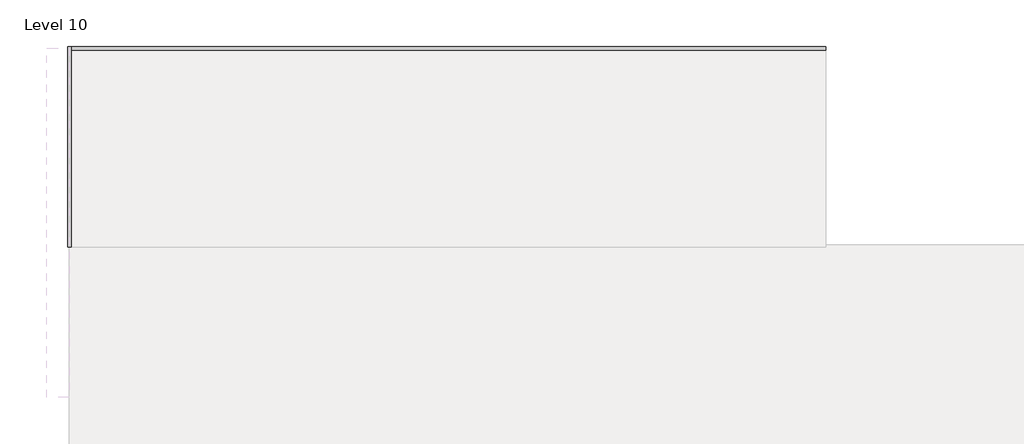
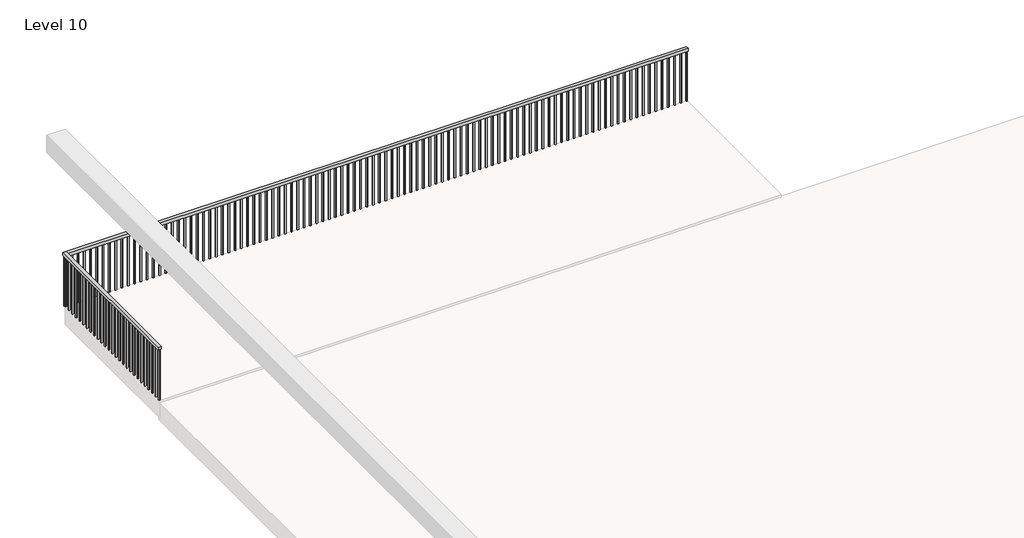
# One storey, part 3 of 5: 2 railings.
"""IFC4 building model written with IfcOpenShell, lengths in millimetres."""

from ifc_helpers import new_model, si_unit, frame, origin, place, context, project, spatial, polyline, outline, extrude, element, save

model = new_model("IFC4")

# Units and contexts
model_context = context("Model", 3, world=origin())
ifc_project = project(units=[si_unit("LENGTHUNIT", "METRE", prefix="MILLI")], contexts=[model_context])

# Site, building, storey
site = spatial("IfcSite", under=ifc_project)
building = spatial("IfcBuilding", under=site)
storey = spatial("IfcBuildingStorey", under=building, Name="Level 10", Elevation=12496.8)

# Railings
placement = place(None, origin())
element("IfcRailing", 1, ObjectType="Handrail - Rectangular", at=placement, inside=storey, context=model_context, shape_type="SweptSolid", body=[
    extrude(outline(polyline([(-13833.4638778, 17386.5959632), (-13833.4638778, 17437.3959632), (-3775.0638778, 17437.3959632), (-3775.0638778, 17386.5959632), (-13833.4638778, 17386.5959632)])), frame((0.0, 0.0, 13360.4), z_axis=(0.0, 0.0, 1.0), x_axis=(1.0, 0.0, 0.0)), (0.0, 0.0, 1.0), 50.8),
    extrude(outline(polyline([(-3886.1888778, 17402.4709632), (-3886.1888778, 17421.5209632), (-3867.1388778, 17421.5209632), (-3867.1388778, 17402.4709632), (-3886.1888778, 17402.4709632)])), frame((0.0, 0.0, 12496.8), z_axis=(0.0, 0.0, 1.0), x_axis=(1.0, 0.0, 0.0)), (0.0, 0.0, 1.0), 863.6),
    extrude(outline(polyline([(-3987.7888778, 17402.4709632), (-3987.7888778, 17421.5209632), (-3968.7388778, 17421.5209632), (-3968.7388778, 17402.4709632), (-3987.7888778, 17402.4709632)])), frame((0.0, 0.0, 12496.8), z_axis=(0.0, 0.0, 1.0), x_axis=(1.0, 0.0, 0.0)), (0.0, 0.0, 1.0), 863.6),
    extrude(outline(polyline([(-4089.3888778, 17402.4709632), (-4089.3888778, 17421.5209632), (-4070.3388778, 17421.5209632), (-4070.3388778, 17402.4709632), (-4089.3888778, 17402.4709632)])), frame((0.0, 0.0, 12496.8), z_axis=(0.0, 0.0, 1.0), x_axis=(1.0, 0.0, 0.0)), (0.0, 0.0, 1.0), 863.6),
    extrude(outline(polyline([(-4190.9888778, 17402.4709632), (-4190.9888778, 17421.5209632), (-4171.9388778, 17421.5209632), (-4171.9388778, 17402.4709632), (-4190.9888778, 17402.4709632)])), frame((0.0, 0.0, 12496.8), z_axis=(0.0, 0.0, 1.0), x_axis=(1.0, 0.0, 0.0)), (0.0, 0.0, 1.0), 863.6),
    extrude(outline(polyline([(-4292.5888778, 17402.4709632), (-4292.5888778, 17421.5209632), (-4273.5388778, 17421.5209632), (-4273.5388778, 17402.4709632), (-4292.5888778, 17402.4709632)])), frame((0.0, 0.0, 12496.8), z_axis=(0.0, 0.0, 1.0), x_axis=(1.0, 0.0, 0.0)), (0.0, 0.0, 1.0), 863.6),
    extrude(outline(polyline([(-4394.1888778, 17402.4709632), (-4394.1888778, 17421.5209632), (-4375.1388778, 17421.5209632), (-4375.1388778, 17402.4709632), (-4394.1888778, 17402.4709632)])), frame((0.0, 0.0, 12496.8), z_axis=(0.0, 0.0, 1.0), x_axis=(1.0, 0.0, 0.0)), (0.0, 0.0, 1.0), 863.6),
    extrude(outline(polyline([(-4495.7888778, 17402.4709632), (-4495.7888778, 17421.5209632), (-4476.7388778, 17421.5209632), (-4476.7388778, 17402.4709632), (-4495.7888778, 17402.4709632)])), frame((0.0, 0.0, 12496.8), z_axis=(0.0, 0.0, 1.0), x_axis=(1.0, 0.0, 0.0)), (0.0, 0.0, 1.0), 863.6),
    extrude(outline(polyline([(-4597.3888778, 17402.4709632), (-4597.3888778, 17421.5209632), (-4578.3388778, 17421.5209632), (-4578.3388778, 17402.4709632), (-4597.3888778, 17402.4709632)])), frame((0.0, 0.0, 12496.8), z_axis=(0.0, 0.0, 1.0), x_axis=(1.0, 0.0, 0.0)), (0.0, 0.0, 1.0), 863.6),
    extrude(outline(polyline([(-4698.9888778, 17402.4709632), (-4698.9888778, 17421.5209632), (-4679.9388778, 17421.5209632), (-4679.9388778, 17402.4709632), (-4698.9888778, 17402.4709632)])), frame((0.0, 0.0, 12496.8), z_axis=(0.0, 0.0, 1.0), x_axis=(1.0, 0.0, 0.0)), (0.0, 0.0, 1.0), 863.6),
    extrude(outline(polyline([(-4800.5888778, 17402.4709632), (-4800.5888778, 17421.5209632), (-4781.5388778, 17421.5209632), (-4781.5388778, 17402.4709632), (-4800.5888778, 17402.4709632)])), frame((0.0, 0.0, 12496.8), z_axis=(0.0, 0.0, 1.0), x_axis=(1.0, 0.0, 0.0)), (0.0, 0.0, 1.0), 863.6),
    extrude(outline(polyline([(-4902.1888778, 17402.4709632), (-4902.1888778, 17421.5209632), (-4883.1388778, 17421.5209632), (-4883.1388778, 17402.4709632), (-4902.1888778, 17402.4709632)])), frame((0.0, 0.0, 12496.8), z_axis=(0.0, 0.0, 1.0), x_axis=(1.0, 0.0, 0.0)), (0.0, 0.0, 1.0), 863.6),
    extrude(outline(polyline([(-5003.7888778, 17402.4709632), (-5003.7888778, 17421.5209632), (-4984.7388778, 17421.5209632), (-4984.7388778, 17402.4709632), (-5003.7888778, 17402.4709632)])), frame((0.0, 0.0, 12496.8), z_axis=(0.0, 0.0, 1.0), x_axis=(1.0, 0.0, 0.0)), (0.0, 0.0, 1.0), 863.6),
    extrude(outline(polyline([(-5105.3888778, 17402.4709632), (-5105.3888778, 17421.5209632), (-5086.3388778, 17421.5209632), (-5086.3388778, 17402.4709632), (-5105.3888778, 17402.4709632)])), frame((0.0, 0.0, 12496.8), z_axis=(0.0, 0.0, 1.0), x_axis=(1.0, 0.0, 0.0)), (0.0, 0.0, 1.0), 863.6),
    extrude(outline(polyline([(-5206.9888778, 17402.4709632), (-5206.9888778, 17421.5209632), (-5187.9388778, 17421.5209632), (-5187.9388778, 17402.4709632), (-5206.9888778, 17402.4709632)])), frame((0.0, 0.0, 12496.8), z_axis=(0.0, 0.0, 1.0), x_axis=(1.0, 0.0, 0.0)), (0.0, 0.0, 1.0), 863.6),
    extrude(outline(polyline([(-5308.5888778, 17402.4709632), (-5308.5888778, 17421.5209632), (-5289.5388778, 17421.5209632), (-5289.5388778, 17402.4709632), (-5308.5888778, 17402.4709632)])), frame((0.0, 0.0, 12496.8), z_axis=(0.0, 0.0, 1.0), x_axis=(1.0, 0.0, 0.0)), (0.0, 0.0, 1.0), 863.6),
    extrude(outline(polyline([(-5410.1888778, 17402.4709632), (-5410.1888778, 17421.5209632), (-5391.1388778, 17421.5209632), (-5391.1388778, 17402.4709632), (-5410.1888778, 17402.4709632)])), frame((0.0, 0.0, 12496.8), z_axis=(0.0, 0.0, 1.0), x_axis=(1.0, 0.0, 0.0)), (0.0, 0.0, 1.0), 863.6),
    extrude(outline(polyline([(-5511.7888778, 17402.4709632), (-5511.7888778, 17421.5209632), (-5492.7388778, 17421.5209632), (-5492.7388778, 17402.4709632), (-5511.7888778, 17402.4709632)])), frame((0.0, 0.0, 12496.8), z_axis=(0.0, 0.0, 1.0), x_axis=(1.0, 0.0, 0.0)), (0.0, 0.0, 1.0), 863.6),
    extrude(outline(polyline([(-5613.3888778, 17402.4709632), (-5613.3888778, 17421.5209632), (-5594.3388778, 17421.5209632), (-5594.3388778, 17402.4709632), (-5613.3888778, 17402.4709632)])), frame((0.0, 0.0, 12496.8), z_axis=(0.0, 0.0, 1.0), x_axis=(1.0, 0.0, 0.0)), (0.0, 0.0, 1.0), 863.6),
    extrude(outline(polyline([(-5714.9888778, 17402.4709632), (-5714.9888778, 17421.5209632), (-5695.9388778, 17421.5209632), (-5695.9388778, 17402.4709632), (-5714.9888778, 17402.4709632)])), frame((0.0, 0.0, 12496.8), z_axis=(0.0, 0.0, 1.0), x_axis=(1.0, 0.0, 0.0)), (0.0, 0.0, 1.0), 863.6),
    extrude(outline(polyline([(-5816.5888778, 17402.4709632), (-5816.5888778, 17421.5209632), (-5797.5388778, 17421.5209632), (-5797.5388778, 17402.4709632), (-5816.5888778, 17402.4709632)])), frame((0.0, 0.0, 12496.8), z_axis=(0.0, 0.0, 1.0), x_axis=(1.0, 0.0, 0.0)), (0.0, 0.0, 1.0), 863.6),
    extrude(outline(polyline([(-5918.1888778, 17402.4709632), (-5918.1888778, 17421.5209632), (-5899.1388778, 17421.5209632), (-5899.1388778, 17402.4709632), (-5918.1888778, 17402.4709632)])), frame((0.0, 0.0, 12496.8), z_axis=(0.0, 0.0, 1.0), x_axis=(1.0, 0.0, 0.0)), (0.0, 0.0, 1.0), 863.6),
    extrude(outline(polyline([(-6019.7888778, 17402.4709632), (-6019.7888778, 17421.5209632), (-6000.7388778, 17421.5209632), (-6000.7388778, 17402.4709632), (-6019.7888778, 17402.4709632)])), frame((0.0, 0.0, 12496.8), z_axis=(0.0, 0.0, 1.0), x_axis=(1.0, 0.0, 0.0)), (0.0, 0.0, 1.0), 863.6),
    extrude(outline(polyline([(-6121.3888778, 17402.4709632), (-6121.3888778, 17421.5209632), (-6102.3388778, 17421.5209632), (-6102.3388778, 17402.4709632), (-6121.3888778, 17402.4709632)])), frame((0.0, 0.0, 12496.8), z_axis=(0.0, 0.0, 1.0), x_axis=(1.0, 0.0, 0.0)), (0.0, 0.0, 1.0), 863.6),
    extrude(outline(polyline([(-6222.9888778, 17402.4709632), (-6222.9888778, 17421.5209632), (-6203.9388778, 17421.5209632), (-6203.9388778, 17402.4709632), (-6222.9888778, 17402.4709632)])), frame((0.0, 0.0, 12496.8), z_axis=(0.0, 0.0, 1.0), x_axis=(1.0, 0.0, 0.0)), (0.0, 0.0, 1.0), 863.6),
    extrude(outline(polyline([(-6324.5888778, 17402.4709632), (-6324.5888778, 17421.5209632), (-6305.5388778, 17421.5209632), (-6305.5388778, 17402.4709632), (-6324.5888778, 17402.4709632)])), frame((0.0, 0.0, 12496.8), z_axis=(0.0, 0.0, 1.0), x_axis=(1.0, 0.0, 0.0)), (0.0, 0.0, 1.0), 863.6),
    extrude(outline(polyline([(-6426.1888778, 17402.4709632), (-6426.1888778, 17421.5209632), (-6407.1388778, 17421.5209632), (-6407.1388778, 17402.4709632), (-6426.1888778, 17402.4709632)])), frame((0.0, 0.0, 12496.8), z_axis=(0.0, 0.0, 1.0), x_axis=(1.0, 0.0, 0.0)), (0.0, 0.0, 1.0), 863.6),
    extrude(outline(polyline([(-6527.7888778, 17402.4709632), (-6527.7888778, 17421.5209632), (-6508.7388778, 17421.5209632), (-6508.7388778, 17402.4709632), (-6527.7888778, 17402.4709632)])), frame((0.0, 0.0, 12496.8), z_axis=(0.0, 0.0, 1.0), x_axis=(1.0, 0.0, 0.0)), (0.0, 0.0, 1.0), 863.6),
    extrude(outline(polyline([(-6629.3888778, 17402.4709632), (-6629.3888778, 17421.5209632), (-6610.3388778, 17421.5209632), (-6610.3388778, 17402.4709632), (-6629.3888778, 17402.4709632)])), frame((0.0, 0.0, 12496.8), z_axis=(0.0, 0.0, 1.0), x_axis=(1.0, 0.0, 0.0)), (0.0, 0.0, 1.0), 863.6),
    extrude(outline(polyline([(-6730.9888778, 17402.4709632), (-6730.9888778, 17421.5209632), (-6711.9388778, 17421.5209632), (-6711.9388778, 17402.4709632), (-6730.9888778, 17402.4709632)])), frame((0.0, 0.0, 12496.8), z_axis=(0.0, 0.0, 1.0), x_axis=(1.0, 0.0, 0.0)), (0.0, 0.0, 1.0), 863.6),
    extrude(outline(polyline([(-6832.5888778, 17402.4709632), (-6832.5888778, 17421.5209632), (-6813.5388778, 17421.5209632), (-6813.5388778, 17402.4709632), (-6832.5888778, 17402.4709632)])), frame((0.0, 0.0, 12496.8), z_axis=(0.0, 0.0, 1.0), x_axis=(1.0, 0.0, 0.0)), (0.0, 0.0, 1.0), 863.6),
    extrude(outline(polyline([(-6934.1888778, 17402.4709632), (-6934.1888778, 17421.5209632), (-6915.1388778, 17421.5209632), (-6915.1388778, 17402.4709632), (-6934.1888778, 17402.4709632)])), frame((0.0, 0.0, 12496.8), z_axis=(0.0, 0.0, 1.0), x_axis=(1.0, 0.0, 0.0)), (0.0, 0.0, 1.0), 863.6),
    extrude(outline(polyline([(-7035.7888778, 17402.4709632), (-7035.7888778, 17421.5209632), (-7016.7388778, 17421.5209632), (-7016.7388778, 17402.4709632), (-7035.7888778, 17402.4709632)])), frame((0.0, 0.0, 12496.8), z_axis=(0.0, 0.0, 1.0), x_axis=(1.0, 0.0, 0.0)), (0.0, 0.0, 1.0), 863.6),
    extrude(outline(polyline([(-7137.3888778, 17402.4709632), (-7137.3888778, 17421.5209632), (-7118.3388778, 17421.5209632), (-7118.3388778, 17402.4709632), (-7137.3888778, 17402.4709632)])), frame((0.0, 0.0, 12496.8), z_axis=(0.0, 0.0, 1.0), x_axis=(1.0, 0.0, 0.0)), (0.0, 0.0, 1.0), 863.6),
    extrude(outline(polyline([(-7238.9888778, 17402.4709632), (-7238.9888778, 17421.5209632), (-7219.9388778, 17421.5209632), (-7219.9388778, 17402.4709632), (-7238.9888778, 17402.4709632)])), frame((0.0, 0.0, 12496.8), z_axis=(0.0, 0.0, 1.0), x_axis=(1.0, 0.0, 0.0)), (0.0, 0.0, 1.0), 863.6),
    extrude(outline(polyline([(-7340.5888778, 17402.4709632), (-7340.5888778, 17421.5209632), (-7321.5388778, 17421.5209632), (-7321.5388778, 17402.4709632), (-7340.5888778, 17402.4709632)])), frame((0.0, 0.0, 12496.8), z_axis=(0.0, 0.0, 1.0), x_axis=(1.0, 0.0, 0.0)), (0.0, 0.0, 1.0), 863.6),
    extrude(outline(polyline([(-7442.1888778, 17402.4709632), (-7442.1888778, 17421.5209632), (-7423.1388778, 17421.5209632), (-7423.1388778, 17402.4709632), (-7442.1888778, 17402.4709632)])), frame((0.0, 0.0, 12496.8), z_axis=(0.0, 0.0, 1.0), x_axis=(1.0, 0.0, 0.0)), (0.0, 0.0, 1.0), 863.6),
    extrude(outline(polyline([(-7543.7888778, 17402.4709632), (-7543.7888778, 17421.5209632), (-7524.7388778, 17421.5209632), (-7524.7388778, 17402.4709632), (-7543.7888778, 17402.4709632)])), frame((0.0, 0.0, 12496.8), z_axis=(0.0, 0.0, 1.0), x_axis=(1.0, 0.0, 0.0)), (0.0, 0.0, 1.0), 863.6),
    extrude(outline(polyline([(-7645.3888778, 17402.4709632), (-7645.3888778, 17421.5209632), (-7626.3388778, 17421.5209632), (-7626.3388778, 17402.4709632), (-7645.3888778, 17402.4709632)])), frame((0.0, 0.0, 12496.8), z_axis=(0.0, 0.0, 1.0), x_axis=(1.0, 0.0, 0.0)), (0.0, 0.0, 1.0), 863.6),
    extrude(outline(polyline([(-7746.9888778, 17402.4709632), (-7746.9888778, 17421.5209632), (-7727.9388778, 17421.5209632), (-7727.9388778, 17402.4709632), (-7746.9888778, 17402.4709632)])), frame((0.0, 0.0, 12496.8), z_axis=(0.0, 0.0, 1.0), x_axis=(1.0, 0.0, 0.0)), (0.0, 0.0, 1.0), 863.6),
    extrude(outline(polyline([(-7848.5888778, 17402.4709632), (-7848.5888778, 17421.5209632), (-7829.5388778, 17421.5209632), (-7829.5388778, 17402.4709632), (-7848.5888778, 17402.4709632)])), frame((0.0, 0.0, 12496.8), z_axis=(0.0, 0.0, 1.0), x_axis=(1.0, 0.0, 0.0)), (0.0, 0.0, 1.0), 863.6),
    extrude(outline(polyline([(-7950.1888778, 17402.4709632), (-7950.1888778, 17421.5209632), (-7931.1388778, 17421.5209632), (-7931.1388778, 17402.4709632), (-7950.1888778, 17402.4709632)])), frame((0.0, 0.0, 12496.8), z_axis=(0.0, 0.0, 1.0), x_axis=(1.0, 0.0, 0.0)), (0.0, 0.0, 1.0), 863.6),
    extrude(outline(polyline([(-8051.7888778, 17402.4709632), (-8051.7888778, 17421.5209632), (-8032.7388778, 17421.5209632), (-8032.7388778, 17402.4709632), (-8051.7888778, 17402.4709632)])), frame((0.0, 0.0, 12496.8), z_axis=(0.0, 0.0, 1.0), x_axis=(1.0, 0.0, 0.0)), (0.0, 0.0, 1.0), 863.6),
    extrude(outline(polyline([(-8153.3888778, 17402.4709632), (-8153.3888778, 17421.5209632), (-8134.3388778, 17421.5209632), (-8134.3388778, 17402.4709632), (-8153.3888778, 17402.4709632)])), frame((0.0, 0.0, 12496.8), z_axis=(0.0, 0.0, 1.0), x_axis=(1.0, 0.0, 0.0)), (0.0, 0.0, 1.0), 863.6),
    extrude(outline(polyline([(-8254.9888778, 17402.4709632), (-8254.9888778, 17421.5209632), (-8235.9388778, 17421.5209632), (-8235.9388778, 17402.4709632), (-8254.9888778, 17402.4709632)])), frame((0.0, 0.0, 12496.8), z_axis=(0.0, 0.0, 1.0), x_axis=(1.0, 0.0, 0.0)), (0.0, 0.0, 1.0), 863.6),
    extrude(outline(polyline([(-8356.5888778, 17402.4709632), (-8356.5888778, 17421.5209632), (-8337.5388778, 17421.5209632), (-8337.5388778, 17402.4709632), (-8356.5888778, 17402.4709632)])), frame((0.0, 0.0, 12496.8), z_axis=(0.0, 0.0, 1.0), x_axis=(1.0, 0.0, 0.0)), (0.0, 0.0, 1.0), 863.6),
    extrude(outline(polyline([(-8458.1888778, 17402.4709632), (-8458.1888778, 17421.5209632), (-8439.1388778, 17421.5209632), (-8439.1388778, 17402.4709632), (-8458.1888778, 17402.4709632)])), frame((0.0, 0.0, 12496.8), z_axis=(0.0, 0.0, 1.0), x_axis=(1.0, 0.0, 0.0)), (0.0, 0.0, 1.0), 863.6),
    extrude(outline(polyline([(-8559.7888778, 17402.4709632), (-8559.7888778, 17421.5209632), (-8540.7388778, 17421.5209632), (-8540.7388778, 17402.4709632), (-8559.7888778, 17402.4709632)])), frame((0.0, 0.0, 12496.8), z_axis=(0.0, 0.0, 1.0), x_axis=(1.0, 0.0, 0.0)), (0.0, 0.0, 1.0), 863.6),
    extrude(outline(polyline([(-8661.3888778, 17402.4709632), (-8661.3888778, 17421.5209632), (-8642.3388778, 17421.5209632), (-8642.3388778, 17402.4709632), (-8661.3888778, 17402.4709632)])), frame((0.0, 0.0, 12496.8), z_axis=(0.0, 0.0, 1.0), x_axis=(1.0, 0.0, 0.0)), (0.0, 0.0, 1.0), 863.6),
    extrude(outline(polyline([(-8762.9888778, 17402.4709632), (-8762.9888778, 17421.5209632), (-8743.9388778, 17421.5209632), (-8743.9388778, 17402.4709632), (-8762.9888778, 17402.4709632)])), frame((0.0, 0.0, 12496.8), z_axis=(0.0, 0.0, 1.0), x_axis=(1.0, 0.0, 0.0)), (0.0, 0.0, 1.0), 863.6),
    extrude(outline(polyline([(-8864.5888778, 17402.4709632), (-8864.5888778, 17421.5209632), (-8845.5388778, 17421.5209632), (-8845.5388778, 17402.4709632), (-8864.5888778, 17402.4709632)])), frame((0.0, 0.0, 12496.8), z_axis=(0.0, 0.0, 1.0), x_axis=(1.0, 0.0, 0.0)), (0.0, 0.0, 1.0), 863.6),
    extrude(outline(polyline([(-8966.1888778, 17402.4709632), (-8966.1888778, 17421.5209632), (-8947.1388778, 17421.5209632), (-8947.1388778, 17402.4709632), (-8966.1888778, 17402.4709632)])), frame((0.0, 0.0, 12496.8), z_axis=(0.0, 0.0, 1.0), x_axis=(1.0, 0.0, 0.0)), (0.0, 0.0, 1.0), 863.6),
    extrude(outline(polyline([(-9067.7888778, 17402.4709632), (-9067.7888778, 17421.5209632), (-9048.7388778, 17421.5209632), (-9048.7388778, 17402.4709632), (-9067.7888778, 17402.4709632)])), frame((0.0, 0.0, 12496.8), z_axis=(0.0, 0.0, 1.0), x_axis=(1.0, 0.0, 0.0)), (0.0, 0.0, 1.0), 863.6),
    extrude(outline(polyline([(-9169.3888778, 17402.4709632), (-9169.3888778, 17421.5209632), (-9150.3388778, 17421.5209632), (-9150.3388778, 17402.4709632), (-9169.3888778, 17402.4709632)])), frame((0.0, 0.0, 12496.8), z_axis=(0.0, 0.0, 1.0), x_axis=(1.0, 0.0, 0.0)), (0.0, 0.0, 1.0), 863.6),
    extrude(outline(polyline([(-9270.9888778, 17402.4709632), (-9270.9888778, 17421.5209632), (-9251.9388778, 17421.5209632), (-9251.9388778, 17402.4709632), (-9270.9888778, 17402.4709632)])), frame((0.0, 0.0, 12496.8), z_axis=(0.0, 0.0, 1.0), x_axis=(1.0, 0.0, 0.0)), (0.0, 0.0, 1.0), 863.6),
    extrude(outline(polyline([(-9372.5888778, 17402.4709632), (-9372.5888778, 17421.5209632), (-9353.5388778, 17421.5209632), (-9353.5388778, 17402.4709632), (-9372.5888778, 17402.4709632)])), frame((0.0, 0.0, 12496.8), z_axis=(0.0, 0.0, 1.0), x_axis=(1.0, 0.0, 0.0)), (0.0, 0.0, 1.0), 863.6),
    extrude(outline(polyline([(-9474.1888778, 17402.4709632), (-9474.1888778, 17421.5209632), (-9455.1388778, 17421.5209632), (-9455.1388778, 17402.4709632), (-9474.1888778, 17402.4709632)])), frame((0.0, 0.0, 12496.8), z_axis=(0.0, 0.0, 1.0), x_axis=(1.0, 0.0, 0.0)), (0.0, 0.0, 1.0), 863.6),
    extrude(outline(polyline([(-9575.7888778, 17402.4709632), (-9575.7888778, 17421.5209632), (-9556.7388778, 17421.5209632), (-9556.7388778, 17402.4709632), (-9575.7888778, 17402.4709632)])), frame((0.0, 0.0, 12496.8), z_axis=(0.0, 0.0, 1.0), x_axis=(1.0, 0.0, 0.0)), (0.0, 0.0, 1.0), 863.6),
    extrude(outline(polyline([(-9677.3888778, 17402.4709632), (-9677.3888778, 17421.5209632), (-9658.3388778, 17421.5209632), (-9658.3388778, 17402.4709632), (-9677.3888778, 17402.4709632)])), frame((0.0, 0.0, 12496.8), z_axis=(0.0, 0.0, 1.0), x_axis=(1.0, 0.0, 0.0)), (0.0, 0.0, 1.0), 863.6),
    extrude(outline(polyline([(-9778.9888778, 17402.4709632), (-9778.9888778, 17421.5209632), (-9759.9388778, 17421.5209632), (-9759.9388778, 17402.4709632), (-9778.9888778, 17402.4709632)])), frame((0.0, 0.0, 12496.8), z_axis=(0.0, 0.0, 1.0), x_axis=(1.0, 0.0, 0.0)), (0.0, 0.0, 1.0), 863.6),
    extrude(outline(polyline([(-9880.5888778, 17402.4709632), (-9880.5888778, 17421.5209632), (-9861.5388778, 17421.5209632), (-9861.5388778, 17402.4709632), (-9880.5888778, 17402.4709632)])), frame((0.0, 0.0, 12496.8), z_axis=(0.0, 0.0, 1.0), x_axis=(1.0, 0.0, 0.0)), (0.0, 0.0, 1.0), 863.6),
    extrude(outline(polyline([(-9982.1888778, 17402.4709632), (-9982.1888778, 17421.5209632), (-9963.1388778, 17421.5209632), (-9963.1388778, 17402.4709632), (-9982.1888778, 17402.4709632)])), frame((0.0, 0.0, 12496.8), z_axis=(0.0, 0.0, 1.0), x_axis=(1.0, 0.0, 0.0)), (0.0, 0.0, 1.0), 863.6),
    extrude(outline(polyline([(-10083.7888778, 17402.4709632), (-10083.7888778, 17421.5209632), (-10064.7388778, 17421.5209632), (-10064.7388778, 17402.4709632), (-10083.7888778, 17402.4709632)])), frame((0.0, 0.0, 12496.8), z_axis=(0.0, 0.0, 1.0), x_axis=(1.0, 0.0, 0.0)), (0.0, 0.0, 1.0), 863.6),
    extrude(outline(polyline([(-10185.3888778, 17402.4709632), (-10185.3888778, 17421.5209632), (-10166.3388778, 17421.5209632), (-10166.3388778, 17402.4709632), (-10185.3888778, 17402.4709632)])), frame((0.0, 0.0, 12496.8), z_axis=(0.0, 0.0, 1.0), x_axis=(1.0, 0.0, 0.0)), (0.0, 0.0, 1.0), 863.6),
    extrude(outline(polyline([(-10286.9888778, 17402.4709632), (-10286.9888778, 17421.5209632), (-10267.9388778, 17421.5209632), (-10267.9388778, 17402.4709632), (-10286.9888778, 17402.4709632)])), frame((0.0, 0.0, 12496.8), z_axis=(0.0, 0.0, 1.0), x_axis=(1.0, 0.0, 0.0)), (0.0, 0.0, 1.0), 863.6),
    extrude(outline(polyline([(-10388.5888778, 17402.4709632), (-10388.5888778, 17421.5209632), (-10369.5388778, 17421.5209632), (-10369.5388778, 17402.4709632), (-10388.5888778, 17402.4709632)])), frame((0.0, 0.0, 12496.8), z_axis=(0.0, 0.0, 1.0), x_axis=(1.0, 0.0, 0.0)), (0.0, 0.0, 1.0), 863.6),
    extrude(outline(polyline([(-10490.1888778, 17402.4709632), (-10490.1888778, 17421.5209632), (-10471.1388778, 17421.5209632), (-10471.1388778, 17402.4709632), (-10490.1888778, 17402.4709632)])), frame((0.0, 0.0, 12496.8), z_axis=(0.0, 0.0, 1.0), x_axis=(1.0, 0.0, 0.0)), (0.0, 0.0, 1.0), 863.6),
    extrude(outline(polyline([(-10591.7888778, 17402.4709632), (-10591.7888778, 17421.5209632), (-10572.7388778, 17421.5209632), (-10572.7388778, 17402.4709632), (-10591.7888778, 17402.4709632)])), frame((0.0, 0.0, 12496.8), z_axis=(0.0, 0.0, 1.0), x_axis=(1.0, 0.0, 0.0)), (0.0, 0.0, 1.0), 863.6),
    extrude(outline(polyline([(-10693.3888778, 17402.4709632), (-10693.3888778, 17421.5209632), (-10674.3388778, 17421.5209632), (-10674.3388778, 17402.4709632), (-10693.3888778, 17402.4709632)])), frame((0.0, 0.0, 12496.8), z_axis=(0.0, 0.0, 1.0), x_axis=(1.0, 0.0, 0.0)), (0.0, 0.0, 1.0), 863.6),
    extrude(outline(polyline([(-10794.9888778, 17402.4709632), (-10794.9888778, 17421.5209632), (-10775.9388778, 17421.5209632), (-10775.9388778, 17402.4709632), (-10794.9888778, 17402.4709632)])), frame((0.0, 0.0, 12496.8), z_axis=(0.0, 0.0, 1.0), x_axis=(1.0, 0.0, 0.0)), (0.0, 0.0, 1.0), 863.6),
    extrude(outline(polyline([(-10896.5888778, 17402.4709632), (-10896.5888778, 17421.5209632), (-10877.5388778, 17421.5209632), (-10877.5388778, 17402.4709632), (-10896.5888778, 17402.4709632)])), frame((0.0, 0.0, 12496.8), z_axis=(0.0, 0.0, 1.0), x_axis=(1.0, 0.0, 0.0)), (0.0, 0.0, 1.0), 863.6),
    extrude(outline(polyline([(-10998.1888778, 17402.4709632), (-10998.1888778, 17421.5209632), (-10979.1388778, 17421.5209632), (-10979.1388778, 17402.4709632), (-10998.1888778, 17402.4709632)])), frame((0.0, 0.0, 12496.8), z_axis=(0.0, 0.0, 1.0), x_axis=(1.0, 0.0, 0.0)), (0.0, 0.0, 1.0), 863.6),
    extrude(outline(polyline([(-11099.7888778, 17402.4709632), (-11099.7888778, 17421.5209632), (-11080.7388778, 17421.5209632), (-11080.7388778, 17402.4709632), (-11099.7888778, 17402.4709632)])), frame((0.0, 0.0, 12496.8), z_axis=(0.0, 0.0, 1.0), x_axis=(1.0, 0.0, 0.0)), (0.0, 0.0, 1.0), 863.6),
    extrude(outline(polyline([(-11201.3888778, 17402.4709632), (-11201.3888778, 17421.5209632), (-11182.3388778, 17421.5209632), (-11182.3388778, 17402.4709632), (-11201.3888778, 17402.4709632)])), frame((0.0, 0.0, 12496.8), z_axis=(0.0, 0.0, 1.0), x_axis=(1.0, 0.0, 0.0)), (0.0, 0.0, 1.0), 863.6),
    extrude(outline(polyline([(-11302.9888778, 17402.4709632), (-11302.9888778, 17421.5209632), (-11283.9388778, 17421.5209632), (-11283.9388778, 17402.4709632), (-11302.9888778, 17402.4709632)])), frame((0.0, 0.0, 12496.8), z_axis=(0.0, 0.0, 1.0), x_axis=(1.0, 0.0, 0.0)), (0.0, 0.0, 1.0), 863.6),
    extrude(outline(polyline([(-11404.5888778, 17402.4709632), (-11404.5888778, 17421.5209632), (-11385.5388778, 17421.5209632), (-11385.5388778, 17402.4709632), (-11404.5888778, 17402.4709632)])), frame((0.0, 0.0, 12496.8), z_axis=(0.0, 0.0, 1.0), x_axis=(1.0, 0.0, 0.0)), (0.0, 0.0, 1.0), 863.6),
    extrude(outline(polyline([(-11506.1888778, 17402.4709632), (-11506.1888778, 17421.5209632), (-11487.1388778, 17421.5209632), (-11487.1388778, 17402.4709632), (-11506.1888778, 17402.4709632)])), frame((0.0, 0.0, 12496.8), z_axis=(0.0, 0.0, 1.0), x_axis=(1.0, 0.0, 0.0)), (0.0, 0.0, 1.0), 863.6),
    extrude(outline(polyline([(-11607.7888778, 17402.4709632), (-11607.7888778, 17421.5209632), (-11588.7388778, 17421.5209632), (-11588.7388778, 17402.4709632), (-11607.7888778, 17402.4709632)])), frame((0.0, 0.0, 12496.8), z_axis=(0.0, 0.0, 1.0), x_axis=(1.0, 0.0, 0.0)), (0.0, 0.0, 1.0), 863.6),
    extrude(outline(polyline([(-11709.3888778, 17402.4709632), (-11709.3888778, 17421.5209632), (-11690.3388778, 17421.5209632), (-11690.3388778, 17402.4709632), (-11709.3888778, 17402.4709632)])), frame((0.0, 0.0, 12496.8), z_axis=(0.0, 0.0, 1.0), x_axis=(1.0, 0.0, 0.0)), (0.0, 0.0, 1.0), 863.6),
    extrude(outline(polyline([(-11810.9888778, 17402.4709632), (-11810.9888778, 17421.5209632), (-11791.9388778, 17421.5209632), (-11791.9388778, 17402.4709632), (-11810.9888778, 17402.4709632)])), frame((0.0, 0.0, 12496.8), z_axis=(0.0, 0.0, 1.0), x_axis=(1.0, 0.0, 0.0)), (0.0, 0.0, 1.0), 863.6),
    extrude(outline(polyline([(-11912.5888778, 17402.4709632), (-11912.5888778, 17421.5209632), (-11893.5388778, 17421.5209632), (-11893.5388778, 17402.4709632), (-11912.5888778, 17402.4709632)])), frame((0.0, 0.0, 12496.8), z_axis=(0.0, 0.0, 1.0), x_axis=(1.0, 0.0, 0.0)), (0.0, 0.0, 1.0), 863.6),
    extrude(outline(polyline([(-12014.1888778, 17402.4709632), (-12014.1888778, 17421.5209632), (-11995.1388778, 17421.5209632), (-11995.1388778, 17402.4709632), (-12014.1888778, 17402.4709632)])), frame((0.0, 0.0, 12496.8), z_axis=(0.0, 0.0, 1.0), x_axis=(1.0, 0.0, 0.0)), (0.0, 0.0, 1.0), 863.6),
    extrude(outline(polyline([(-12115.7888778, 17402.4709632), (-12115.7888778, 17421.5209632), (-12096.7388778, 17421.5209632), (-12096.7388778, 17402.4709632), (-12115.7888778, 17402.4709632)])), frame((0.0, 0.0, 12496.8), z_axis=(0.0, 0.0, 1.0), x_axis=(1.0, 0.0, 0.0)), (0.0, 0.0, 1.0), 863.6),
    extrude(outline(polyline([(-12217.3888778, 17402.4709632), (-12217.3888778, 17421.5209632), (-12198.3388778, 17421.5209632), (-12198.3388778, 17402.4709632), (-12217.3888778, 17402.4709632)])), frame((0.0, 0.0, 12496.8), z_axis=(0.0, 0.0, 1.0), x_axis=(1.0, 0.0, 0.0)), (0.0, 0.0, 1.0), 863.6),
    extrude(outline(polyline([(-12318.9888778, 17402.4709632), (-12318.9888778, 17421.5209632), (-12299.9388778, 17421.5209632), (-12299.9388778, 17402.4709632), (-12318.9888778, 17402.4709632)])), frame((0.0, 0.0, 12496.8), z_axis=(0.0, 0.0, 1.0), x_axis=(1.0, 0.0, 0.0)), (0.0, 0.0, 1.0), 863.6),
    extrude(outline(polyline([(-12420.5888778, 17402.4709632), (-12420.5888778, 17421.5209632), (-12401.5388778, 17421.5209632), (-12401.5388778, 17402.4709632), (-12420.5888778, 17402.4709632)])), frame((0.0, 0.0, 12496.8), z_axis=(0.0, 0.0, 1.0), x_axis=(1.0, 0.0, 0.0)), (0.0, 0.0, 1.0), 863.6),
    extrude(outline(polyline([(-12522.1888778, 17402.4709632), (-12522.1888778, 17421.5209632), (-12503.1388778, 17421.5209632), (-12503.1388778, 17402.4709632), (-12522.1888778, 17402.4709632)])), frame((0.0, 0.0, 12496.8), z_axis=(0.0, 0.0, 1.0), x_axis=(1.0, 0.0, 0.0)), (0.0, 0.0, 1.0), 863.6),
    extrude(outline(polyline([(-12623.7888778, 17402.4709632), (-12623.7888778, 17421.5209632), (-12604.7388778, 17421.5209632), (-12604.7388778, 17402.4709632), (-12623.7888778, 17402.4709632)])), frame((0.0, 0.0, 12496.8), z_axis=(0.0, 0.0, 1.0), x_axis=(1.0, 0.0, 0.0)), (0.0, 0.0, 1.0), 863.6),
    extrude(outline(polyline([(-12725.3888778, 17402.4709632), (-12725.3888778, 17421.5209632), (-12706.3388778, 17421.5209632), (-12706.3388778, 17402.4709632), (-12725.3888778, 17402.4709632)])), frame((0.0, 0.0, 12496.8), z_axis=(0.0, 0.0, 1.0), x_axis=(1.0, 0.0, 0.0)), (0.0, 0.0, 1.0), 863.6),
    extrude(outline(polyline([(-12826.9888778, 17402.4709632), (-12826.9888778, 17421.5209632), (-12807.9388778, 17421.5209632), (-12807.9388778, 17402.4709632), (-12826.9888778, 17402.4709632)])), frame((0.0, 0.0, 12496.8), z_axis=(0.0, 0.0, 1.0), x_axis=(1.0, 0.0, 0.0)), (0.0, 0.0, 1.0), 863.6),
    extrude(outline(polyline([(-12928.5888778, 17402.4709632), (-12928.5888778, 17421.5209632), (-12909.5388778, 17421.5209632), (-12909.5388778, 17402.4709632), (-12928.5888778, 17402.4709632)])), frame((0.0, 0.0, 12496.8), z_axis=(0.0, 0.0, 1.0), x_axis=(1.0, 0.0, 0.0)), (0.0, 0.0, 1.0), 863.6),
    extrude(outline(polyline([(-13030.1888778, 17402.4709632), (-13030.1888778, 17421.5209632), (-13011.1388778, 17421.5209632), (-13011.1388778, 17402.4709632), (-13030.1888778, 17402.4709632)])), frame((0.0, 0.0, 12496.8), z_axis=(0.0, 0.0, 1.0), x_axis=(1.0, 0.0, 0.0)), (0.0, 0.0, 1.0), 863.6),
    extrude(outline(polyline([(-13131.7888778, 17402.4709632), (-13131.7888778, 17421.5209632), (-13112.7388778, 17421.5209632), (-13112.7388778, 17402.4709632), (-13131.7888778, 17402.4709632)])), frame((0.0, 0.0, 12496.8), z_axis=(0.0, 0.0, 1.0), x_axis=(1.0, 0.0, 0.0)), (0.0, 0.0, 1.0), 863.6),
    extrude(outline(polyline([(-13233.3888778, 17402.4709632), (-13233.3888778, 17421.5209632), (-13214.3388778, 17421.5209632), (-13214.3388778, 17402.4709632), (-13233.3888778, 17402.4709632)])), frame((0.0, 0.0, 12496.8), z_axis=(0.0, 0.0, 1.0), x_axis=(1.0, 0.0, 0.0)), (0.0, 0.0, 1.0), 863.6),
    extrude(outline(polyline([(-13334.9888778, 17402.4709632), (-13334.9888778, 17421.5209632), (-13315.9388778, 17421.5209632), (-13315.9388778, 17402.4709632), (-13334.9888778, 17402.4709632)])), frame((0.0, 0.0, 12496.8), z_axis=(0.0, 0.0, 1.0), x_axis=(1.0, 0.0, 0.0)), (0.0, 0.0, 1.0), 863.6),
    extrude(outline(polyline([(-13436.5888778, 17402.4709632), (-13436.5888778, 17421.5209632), (-13417.5388778, 17421.5209632), (-13417.5388778, 17402.4709632), (-13436.5888778, 17402.4709632)])), frame((0.0, 0.0, 12496.8), z_axis=(0.0, 0.0, 1.0), x_axis=(1.0, 0.0, 0.0)), (0.0, 0.0, 1.0), 863.6),
    extrude(outline(polyline([(-13538.1888778, 17402.4709632), (-13538.1888778, 17421.5209632), (-13519.1388778, 17421.5209632), (-13519.1388778, 17402.4709632), (-13538.1888778, 17402.4709632)])), frame((0.0, 0.0, 12496.8), z_axis=(0.0, 0.0, 1.0), x_axis=(1.0, 0.0, 0.0)), (0.0, 0.0, 1.0), 863.6),
    extrude(outline(polyline([(-13639.7888778, 17402.4709632), (-13639.7888778, 17421.5209632), (-13620.7388778, 17421.5209632), (-13620.7388778, 17402.4709632), (-13639.7888778, 17402.4709632)])), frame((0.0, 0.0, 12496.8), z_axis=(0.0, 0.0, 1.0), x_axis=(1.0, 0.0, 0.0)), (0.0, 0.0, 1.0), 863.6),
    extrude(outline(polyline([(-13741.3888778, 17402.4709632), (-13741.3888778, 17421.5209632), (-13722.3388778, 17421.5209632), (-13722.3388778, 17402.4709632), (-13741.3888778, 17402.4709632)])), frame((0.0, 0.0, 12496.8), z_axis=(0.0, 0.0, 1.0), x_axis=(1.0, 0.0, 0.0)), (0.0, 0.0, 1.0), 863.6),
    extrude(outline(polyline([(-3794.1138778, 17402.4709632), (-3794.1138778, 17421.5209632), (-3775.0638778, 17421.5209632), (-3775.0638778, 17402.4709632), (-3794.1138778, 17402.4709632)])), frame((0.0, 0.0, 12496.8), z_axis=(0.0, 0.0, 1.0), x_axis=(1.0, 0.0, 0.0)), (0.0, 0.0, 1.0), 863.6),
    extrude(outline(polyline([(-13833.4638778, 17402.4709632), (-13833.4638778, 17421.5209632), (-13814.4138778, 17421.5209632), (-13814.4138778, 17402.4709632), (-13833.4638778, 17402.4709632)])), frame((0.0, 0.0, 12496.8), z_axis=(0.0, 0.0, 1.0), x_axis=(1.0, 0.0, 0.0)), (0.0, 0.0, 1.0), 863.6),
])
element("IfcRailing", 2, ObjectType="Handrail - Rectangular", at=placement, inside=storey, context=model_context, shape_type="SweptSolid", body=[
    extrude(outline(polyline([(-13808.0638778, 14768.6237525), (-13858.8638778, 14768.6237525), (-13858.8638778, 17437.3959632), (-13808.0638778, 17437.3959632), (-13808.0638778, 14768.6237525)])), frame((0.0, 0.0, 13360.4), z_axis=(0.0, 0.0, 1.0), x_axis=(1.0, 0.0, 0.0)), (0.0, 0.0, 1.0), 50.8),
    extrude(outline(polyline([(-13823.9388778, 17400.6987525), (-13842.9888778, 17400.6987525), (-13842.9888778, 17419.7487525), (-13823.9388778, 17419.7487525), (-13823.9388778, 17400.6987525)])), frame((0.0, 0.0, 12496.8), z_axis=(0.0, 0.0, 1.0), x_axis=(1.0, 0.0, 0.0)), (0.0, 0.0, 1.0), 863.6),
    extrude(outline(polyline([(-13823.9388778, 17299.0987525), (-13842.9888778, 17299.0987525), (-13842.9888778, 17318.1487525), (-13823.9388778, 17318.1487525), (-13823.9388778, 17299.0987525)])), frame((0.0, 0.0, 12496.8), z_axis=(0.0, 0.0, 1.0), x_axis=(1.0, 0.0, 0.0)), (0.0, 0.0, 1.0), 863.6),
    extrude(outline(polyline([(-13823.9388778, 17197.4987525), (-13842.9888778, 17197.4987525), (-13842.9888778, 17216.5487525), (-13823.9388778, 17216.5487525), (-13823.9388778, 17197.4987525)])), frame((0.0, 0.0, 12496.8), z_axis=(0.0, 0.0, 1.0), x_axis=(1.0, 0.0, 0.0)), (0.0, 0.0, 1.0), 863.6),
    extrude(outline(polyline([(-13823.9388778, 17095.8987525), (-13842.9888778, 17095.8987525), (-13842.9888778, 17114.9487525), (-13823.9388778, 17114.9487525), (-13823.9388778, 17095.8987525)])), frame((0.0, 0.0, 12496.8), z_axis=(0.0, 0.0, 1.0), x_axis=(1.0, 0.0, 0.0)), (0.0, 0.0, 1.0), 863.6),
    extrude(outline(polyline([(-13823.9388778, 16994.2987525), (-13842.9888778, 16994.2987525), (-13842.9888778, 17013.3487525), (-13823.9388778, 17013.3487525), (-13823.9388778, 16994.2987525)])), frame((0.0, 0.0, 12496.8), z_axis=(0.0, 0.0, 1.0), x_axis=(1.0, 0.0, 0.0)), (0.0, 0.0, 1.0), 863.6),
    extrude(outline(polyline([(-13823.9388778, 16892.6987525), (-13842.9888778, 16892.6987525), (-13842.9888778, 16911.7487525), (-13823.9388778, 16911.7487525), (-13823.9388778, 16892.6987525)])), frame((0.0, 0.0, 12496.8), z_axis=(0.0, 0.0, 1.0), x_axis=(1.0, 0.0, 0.0)), (0.0, 0.0, 1.0), 863.6),
    extrude(outline(polyline([(-13823.9388778, 16791.0987525), (-13842.9888778, 16791.0987525), (-13842.9888778, 16810.1487525), (-13823.9388778, 16810.1487525), (-13823.9388778, 16791.0987525)])), frame((0.0, 0.0, 12496.8), z_axis=(0.0, 0.0, 1.0), x_axis=(1.0, 0.0, 0.0)), (0.0, 0.0, 1.0), 863.6),
    extrude(outline(polyline([(-13823.9388778, 16689.4987525), (-13842.9888778, 16689.4987525), (-13842.9888778, 16708.5487525), (-13823.9388778, 16708.5487525), (-13823.9388778, 16689.4987525)])), frame((0.0, 0.0, 12496.8), z_axis=(0.0, 0.0, 1.0), x_axis=(1.0, 0.0, 0.0)), (0.0, 0.0, 1.0), 863.6),
    extrude(outline(polyline([(-13823.9388778, 16587.8987525), (-13842.9888778, 16587.8987525), (-13842.9888778, 16606.9487525), (-13823.9388778, 16606.9487525), (-13823.9388778, 16587.8987525)])), frame((0.0, 0.0, 12496.8), z_axis=(0.0, 0.0, 1.0), x_axis=(1.0, 0.0, 0.0)), (0.0, 0.0, 1.0), 863.6),
    extrude(outline(polyline([(-13823.9388778, 16486.2987525), (-13842.9888778, 16486.2987525), (-13842.9888778, 16505.3487525), (-13823.9388778, 16505.3487525), (-13823.9388778, 16486.2987525)])), frame((0.0, 0.0, 12496.8), z_axis=(0.0, 0.0, 1.0), x_axis=(1.0, 0.0, 0.0)), (0.0, 0.0, 1.0), 863.6),
    extrude(outline(polyline([(-13823.9388778, 16384.6987525), (-13842.9888778, 16384.6987525), (-13842.9888778, 16403.7487525), (-13823.9388778, 16403.7487525), (-13823.9388778, 16384.6987525)])), frame((0.0, 0.0, 12496.8), z_axis=(0.0, 0.0, 1.0), x_axis=(1.0, 0.0, 0.0)), (0.0, 0.0, 1.0), 863.6),
    extrude(outline(polyline([(-13823.9388778, 16283.0987525), (-13842.9888778, 16283.0987525), (-13842.9888778, 16302.1487525), (-13823.9388778, 16302.1487525), (-13823.9388778, 16283.0987525)])), frame((0.0, 0.0, 12496.8), z_axis=(0.0, 0.0, 1.0), x_axis=(1.0, 0.0, 0.0)), (0.0, 0.0, 1.0), 863.6),
    extrude(outline(polyline([(-13823.9388778, 16181.4987525), (-13842.9888778, 16181.4987525), (-13842.9888778, 16200.5487525), (-13823.9388778, 16200.5487525), (-13823.9388778, 16181.4987525)])), frame((0.0, 0.0, 12496.8), z_axis=(0.0, 0.0, 1.0), x_axis=(1.0, 0.0, 0.0)), (0.0, 0.0, 1.0), 863.6),
    extrude(outline(polyline([(-13823.9388778, 16079.8987525), (-13842.9888778, 16079.8987525), (-13842.9888778, 16098.9487525), (-13823.9388778, 16098.9487525), (-13823.9388778, 16079.8987525)])), frame((0.0, 0.0, 12496.8), z_axis=(0.0, 0.0, 1.0), x_axis=(1.0, 0.0, 0.0)), (0.0, 0.0, 1.0), 863.6),
    extrude(outline(polyline([(-13823.9388778, 15978.2987525), (-13842.9888778, 15978.2987525), (-13842.9888778, 15997.3487525), (-13823.9388778, 15997.3487525), (-13823.9388778, 15978.2987525)])), frame((0.0, 0.0, 12496.8), z_axis=(0.0, 0.0, 1.0), x_axis=(1.0, 0.0, 0.0)), (0.0, 0.0, 1.0), 863.6),
    extrude(outline(polyline([(-13823.9388778, 15876.6987525), (-13842.9888778, 15876.6987525), (-13842.9888778, 15895.7487525), (-13823.9388778, 15895.7487525), (-13823.9388778, 15876.6987525)])), frame((0.0, 0.0, 12496.8), z_axis=(0.0, 0.0, 1.0), x_axis=(1.0, 0.0, 0.0)), (0.0, 0.0, 1.0), 863.6),
    extrude(outline(polyline([(-13823.9388778, 15775.0987525), (-13842.9888778, 15775.0987525), (-13842.9888778, 15794.1487525), (-13823.9388778, 15794.1487525), (-13823.9388778, 15775.0987525)])), frame((0.0, 0.0, 12496.8), z_axis=(0.0, 0.0, 1.0), x_axis=(1.0, 0.0, 0.0)), (0.0, 0.0, 1.0), 863.6),
    extrude(outline(polyline([(-13823.9388778, 15673.4987525), (-13842.9888778, 15673.4987525), (-13842.9888778, 15692.5487525), (-13823.9388778, 15692.5487525), (-13823.9388778, 15673.4987525)])), frame((0.0, 0.0, 12496.8), z_axis=(0.0, 0.0, 1.0), x_axis=(1.0, 0.0, 0.0)), (0.0, 0.0, 1.0), 863.6),
    extrude(outline(polyline([(-13823.9388778, 15571.8987525), (-13842.9888778, 15571.8987525), (-13842.9888778, 15590.9487525), (-13823.9388778, 15590.9487525), (-13823.9388778, 15571.8987525)])), frame((0.0, 0.0, 12496.8), z_axis=(0.0, 0.0, 1.0), x_axis=(1.0, 0.0, 0.0)), (0.0, 0.0, 1.0), 863.6),
    extrude(outline(polyline([(-13823.9388778, 15470.2987525), (-13842.9888778, 15470.2987525), (-13842.9888778, 15489.3487525), (-13823.9388778, 15489.3487525), (-13823.9388778, 15470.2987525)])), frame((0.0, 0.0, 12496.8), z_axis=(0.0, 0.0, 1.0), x_axis=(1.0, 0.0, 0.0)), (0.0, 0.0, 1.0), 863.6),
    extrude(outline(polyline([(-13823.9388778, 15368.6987525), (-13842.9888778, 15368.6987525), (-13842.9888778, 15387.7487525), (-13823.9388778, 15387.7487525), (-13823.9388778, 15368.6987525)])), frame((0.0, 0.0, 12496.8), z_axis=(0.0, 0.0, 1.0), x_axis=(1.0, 0.0, 0.0)), (0.0, 0.0, 1.0), 863.6),
    extrude(outline(polyline([(-13823.9388778, 15267.0987525), (-13842.9888778, 15267.0987525), (-13842.9888778, 15286.1487525), (-13823.9388778, 15286.1487525), (-13823.9388778, 15267.0987525)])), frame((0.0, 0.0, 12496.8), z_axis=(0.0, 0.0, 1.0), x_axis=(1.0, 0.0, 0.0)), (0.0, 0.0, 1.0), 863.6),
    extrude(outline(polyline([(-13823.9388778, 15165.4987525), (-13842.9888778, 15165.4987525), (-13842.9888778, 15184.5487525), (-13823.9388778, 15184.5487525), (-13823.9388778, 15165.4987525)])), frame((0.0, 0.0, 12496.8), z_axis=(0.0, 0.0, 1.0), x_axis=(1.0, 0.0, 0.0)), (0.0, 0.0, 1.0), 863.6),
    extrude(outline(polyline([(-13823.9388778, 15063.8987525), (-13842.9888778, 15063.8987525), (-13842.9888778, 15082.9487525), (-13823.9388778, 15082.9487525), (-13823.9388778, 15063.8987525)])), frame((0.0, 0.0, 12496.8), z_axis=(0.0, 0.0, 1.0), x_axis=(1.0, 0.0, 0.0)), (0.0, 0.0, 1.0), 863.6),
    extrude(outline(polyline([(-13823.9388778, 14962.2987525), (-13842.9888778, 14962.2987525), (-13842.9888778, 14981.3487525), (-13823.9388778, 14981.3487525), (-13823.9388778, 14962.2987525)])), frame((0.0, 0.0, 12496.8), z_axis=(0.0, 0.0, 1.0), x_axis=(1.0, 0.0, 0.0)), (0.0, 0.0, 1.0), 863.6),
    extrude(outline(polyline([(-13823.9388778, 14860.6987525), (-13842.9888778, 14860.6987525), (-13842.9888778, 14879.7487525), (-13823.9388778, 14879.7487525), (-13823.9388778, 14860.6987525)])), frame((0.0, 0.0, 12496.8), z_axis=(0.0, 0.0, 1.0), x_axis=(1.0, 0.0, 0.0)), (0.0, 0.0, 1.0), 863.6),
    extrude(outline(polyline([(-13823.9388778, 17418.3459632), (-13842.9888778, 17418.3459632), (-13842.9888778, 17437.3959632), (-13823.9388778, 17437.3959632), (-13823.9388778, 17418.3459632)])), frame((0.0, 0.0, 12496.8), z_axis=(0.0, 0.0, 1.0), x_axis=(1.0, 0.0, 0.0)), (0.0, 0.0, 1.0), 863.6),
    extrude(outline(polyline([(-13823.9388778, 14768.6237525), (-13842.9888778, 14768.6237525), (-13842.9888778, 14787.6737525), (-13823.9388778, 14787.6737525), (-13823.9388778, 14768.6237525)])), frame((0.0, 0.0, 12496.8), z_axis=(0.0, 0.0, 1.0), x_axis=(1.0, 0.0, 0.0)), (0.0, 0.0, 1.0), 863.6),
])

save(model, "model.ifc")

# Revit data of these elements
# Type "Handrail - Rectangular"
#   Assembly Code = "C2010400"
#   built-in parameter 1008612 = 0.0416667 (stored number, unit not read)
#   built-in parameter 1008611 = 0.0416667 (stored number, unit not read)
#   built-in parameter 1008609 = 0.333333 (stored number, unit not read)
#   built-in parameter 1008604 = 0.166667 (stored number, unit not read)
#   built-in parameter 1008603 = 0.166667 (stored number, unit not read)
#   Railing Height = 3' - 0"
#   built-in parameter 1008630 = 2
#   built-in parameter 1008610 = 2
#   built-in parameter 1008618 = Baluster - Square : 3/4"
# Elements 1, 2 (IfcRailing, "Handrail - Rectangular")
#   Phase Created = New Construction
